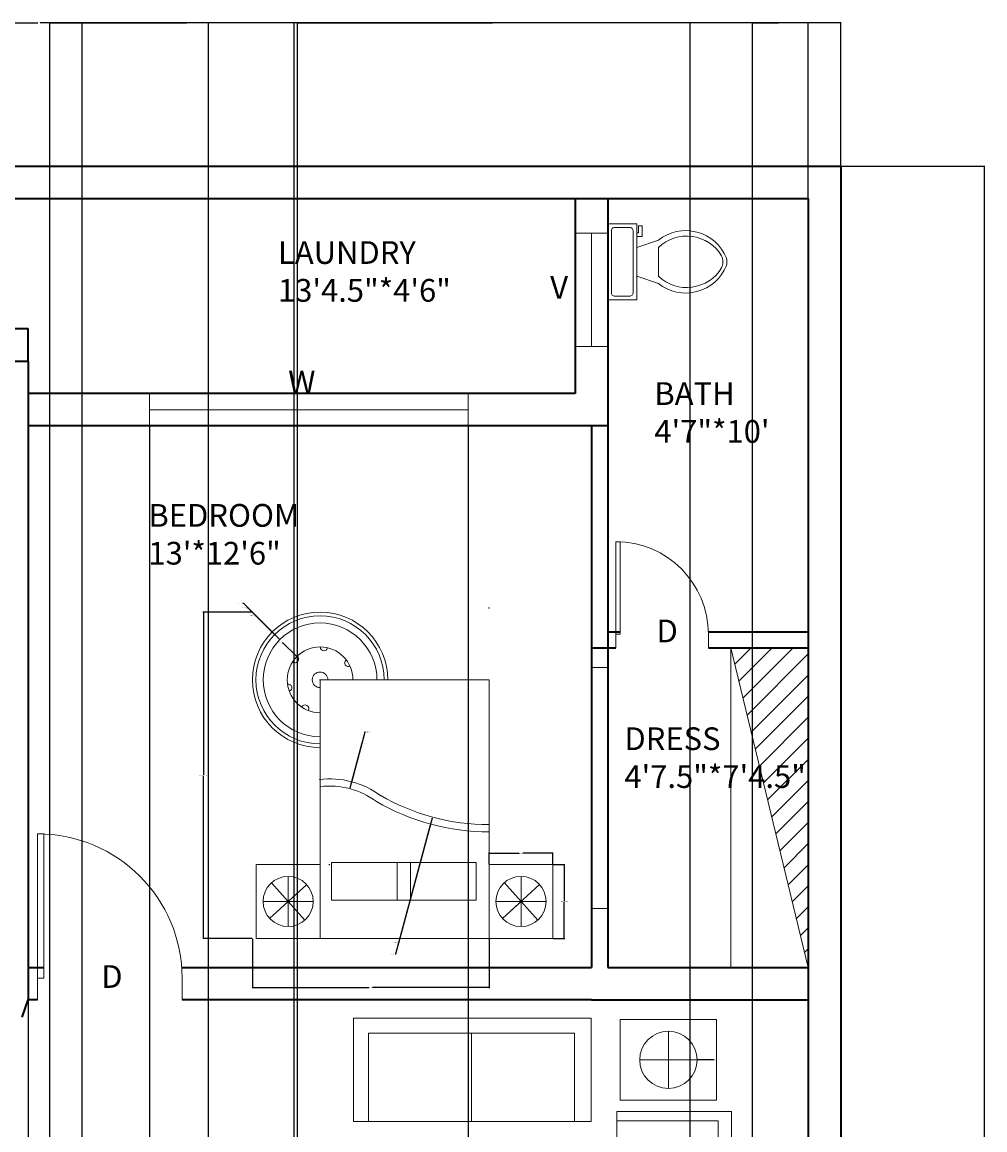
# Model space of a CAD drawing. Units: inches. Extents: x 2284 to 2815, y 1123 to 1948.
# Tile 6 of 6: x 2548 to 2814, y 1641 to 1948. Entities that reach past the tile are written whole.
import ezdxf

# ---------------------------------------------------------------- set-up
doc = ezdxf.new("R2010")
doc.units = ezdxf.units.IN
for name, color, linetype, lineweight in [('A-ANNO-DIMS', 2, 'Continuous', 18), ('A-AREA-IDEN', 30, 'Continuous', 18), ('A-CASE-PATT', 217, 'Continuous', 13), ('A-FLOR-CASE', 8, 'Continuous', 18), ('A-FLOR-FIXT', 9, 'Continuous', 18), ('A-WALL-PATT', 140, 'Continuous', 13), ('C-SITE-WALL', 7, 'Continuous', 35), ('DOOR', 190, 'Continuous', 18), ('FUR', 10, 'Continuous', 18), ('TEXT', 30, 'Continuous', 18), ('WALL', 7, 'Continuous', 35), ('WIND', 210, 'Continuous', 18)]:
    doc.layers.add(name, color=color, linetype=linetype, lineweight=lineweight)
doc.styles.get("Standard").update_dxf_attribs({"font": 'arial.ttf'})
doc.dimstyles.get("Standard").update_dxf_attribs({"dimtxt": 0.18, "dimasz": 0.18, "dimexe": 0.18, "dimexo": 0.0625, "dimgap": 0.09, "dimtad": 0, "dimtih": 1, "dimtoh": 1, "dimdec": 4, "dimzin": 0, "dimdsep": 46, "dimtxsty": 'Standard', "dimcen": 0.09, "dimadec": 0, "dimazin": 0, "dimtfac": 1, "dimtdec": 4, "dimtofl": 0, "dimtmove": 0, "dimatfit": 3, "dimfxl": 1, "dimtolj": 1, "dimtzin": 0, "dimarcsym": 0})

# ---------------------------------------------------------------- blocks, each defined once
blk = doc.blocks.new('*U2')
for p, q in [((0, 0), (0, -6)), ((40, 0), (40, -6))]:
    blk.add_line(p, q)
blk.add_lwpolyline([(0, 0), (0, 40), (1.75, 40), (1.75, 0)], close=True)
blk.add_arc((0, 0), 40, 0, 90)
blk = doc.blocks.new('*U4')
for p, q in [((9.5, -6), (9.5, -2)), ((-10, -8.5), (-8, -8.5)), ((-10, -9.5), (-10, -8.5)), ((-8, -8.5), (-8, -8)), ((-7, -8), (-7, -9.5)), ((-4, -8), (-6, -14)), ((4, -8), (6, -14)), ((-7, -9.5), (-10, -9.5)), ((4, -14), (-4, -14))]:
    blk.add_line(p, q)
blk.add_lwpolyline([(10.5, -8), (10.5, 0), (-10.5, 0), (-10.5, -8)], close=True)
for points in [[(-9.5, -2), (-9.5, -6)], [(8.5, -1), (-8.5, -1)], [(-8.5, -7), (8.5, -7)]]:
    blk.add_lwpolyline(points)
for centre, radius, start, end in [((-8.62, -1.88), 0.884, 81.8699, 188.1301), ((8.62, -1.88), 0.884, 351.8699, 98.1301), ((-8.62, -6.12), 0.884, 171.8699, 278.1301), ((8.62, -6.12), 0.884, 261.8699, 8.1301), ((3.52, -21.58), 12.17, 141.4691, 247.9714), ((4.2, -21.82), 11.33, 136.3677, 238.9468), ((-3.52, -21.58), 12.17, 292.0284, 38.5307), ((-4.2, -21.82), 11.33, 301.053, 43.6321), ((0, -27.88), 4, 245.7318, 294.2682), ((0, -29), 4, 254.8605, 285.1395)]:
    blk.add_arc(centre, radius, start, end)
blk = doc.blocks.new('BED-DOUBLE-WITH-RUG')
for points in [[(0, 0), (71.68, 0), (71.68, 46.8), (0, 46.8)], [(10.67, 21.75), (21.03, 21.75), (21.03, 43.61), (10.67, 43.61)], [(10.67, 3.58), (21.03, 3.58), (21.03, 25.43), (10.67, 25.43)]]:
    blk.add_lwpolyline(points, close=True)
for centre, radius, start, end in [((71.68, 46.8), 18.75, 270, 180), ((71.68, 46.8), 17.75, 270, 180), ((71.68, 46.8), 15.75, 270, 180), ((71.68, 46.8), 9.1, 270, 180), ((69.48, 55.63), 1, 197.1257, 10.8048), ((77.45, 53.83), 1.1, 144.137, 317.2027), ((63.62, 51.01), 1.12, 245.9164, 58.891), ((20.54, 44.16), 21.72, 323.3068, 6.9612), ((20.54, 44.16), 23.72, 323.3068, 6.9612), ((71.68, 46.8), 2.16, 270, 180), ((80.72, 45.75), 0.986, 86.4879, 260.2794), ((76.34, 38.98), 1, 33.9622, 207.6652), ((91.6, 0), 62.04, 149.8305, 180), ((91.6, 0), 60.04, 149.8305, 180)]:
    blk.add_arc(centre, radius, start, end)
blk = doc.blocks.new('NIGHTSTAND-LAMP')
for p, q in [((10.28, 1.89), (10.28, 15.8)), ((15.48, 13.46), (5.08, 4.23)), ((10.28, 8.85), (5.59, 13.98)), ((5.59, 13.98), (14.97, 3.71)), ((10.28, 8.85), (15.48, 13.46)), ((3.33, 8.85), (17.23, 8.85))]:
    blk.add_line(p, q)
blk.add_lwpolyline([(0, 0), (20.56, 0), (20.56, 17.69), (0, 17.69)], close=True)
blk.add_circle((10.28, 8.85), 6.95)
blk = doc.blocks.new('*D14')
at = {"layer": 'A-ANNO-DIMS', "color": 0, "lineweight": -2, "transparency": 16777216}
for p, q in [((2611.59, 1784.82), (2597.91, 1784.82)), ((2598.09, 1784.64), (2598.09, 1739.79)), ((2598.09, 1694.58), (2598.09, 1739.43)), ((2611.59, 1694.4), (2597.91, 1694.4))]:
    blk.add_line(p, q, dxfattribs=at)
at = {"layer": 'A-ANNO-DIMS', "color": 0, "transparency": 16777216}
for points in [[(2598.06, 1784.64), (2598.12, 1784.64), (2598.09, 1784.82)], [(2598.06, 1694.58), (2598.12, 1694.58), (2598.09, 1694.4)]]:
    blk.add_solid(points, dxfattribs=at)
at = {"layer": 'Defpoints', "color": 0, "transparency": 16777216}
for p in [(2598.09, 1784.82), (2611.65, 1784.82), (2611.65, 1694.4)]:
    blk.add_point(p, dxfattribs=at)
at = {"layer": 'A-ANNO-DIMS', "color": 0, "transparency": 16777216, "insert": (2598.09, 1739.61), "char_height": 0.18, "attachment_point": 5}
blk.add_mtext('\\A1;BED / RUG 90 TYP.', dxfattribs=at)
blk = doc.blocks.new('*D15')
at = {"layer": 'A-ANNO-DIMS', "color": 0, "lineweight": -2, "transparency": 16777216}
for p, q in [((2611.65, 1694.33), (2611.65, 1680.65)), ((2677.19, 1694.33), (2677.19, 1680.65)), ((2611.83, 1680.83), (2643.89, 1680.83)), ((2677.01, 1680.83), (2644.95, 1680.83))]:
    blk.add_line(p, q, dxfattribs=at)
at = {"layer": 'A-ANNO-DIMS', "color": 0, "transparency": 16777216}
for points in [[(2611.83, 1680.86), (2611.83, 1680.8), (2611.65, 1680.83)], [(2677.01, 1680.86), (2677.01, 1680.8), (2677.19, 1680.83)]]:
    blk.add_solid(points, dxfattribs=at)
at = {"layer": 'Defpoints', "color": 0, "transparency": 16777216}
for p in [(2611.65, 1694.4), (2677.19, 1694.4), (2611.65, 1680.83)]:
    blk.add_point(p, dxfattribs=at)
at = {"layer": 'A-ANNO-DIMS', "color": 0, "transparency": 16777216, "insert": (2644.42, 1680.83), "char_height": 0.18, "attachment_point": 5}
blk.add_mtext('\\A1;66 TYP.', dxfattribs=at)
blk = doc.blocks.new('*D16')
at = {"layer": 'A-ANNO-DIMS', "color": 0, "lineweight": -2, "transparency": 16777216}
for p, q in [((2694.94, 1714.96), (2698.15, 1714.96)), ((2697.97, 1714.78), (2697.97, 1704.86)), ((2697.97, 1694.58), (2697.97, 1704.49)), ((2694.94, 1694.4), (2698.15, 1694.4))]:
    blk.add_line(p, q, dxfattribs=at)
at = {"layer": 'A-ANNO-DIMS', "color": 0, "transparency": 16777216}
for points in [[(2697.94, 1714.78), (2698, 1714.78), (2697.97, 1714.96)], [(2697.94, 1694.58), (2698, 1694.58), (2697.97, 1694.4)]]:
    blk.add_solid(points, dxfattribs=at)
at = {"layer": 'Defpoints', "color": 0, "transparency": 16777216}
for p in [(2694.88, 1714.96), (2697.97, 1714.96), (2694.88, 1694.4)]:
    blk.add_point(p, dxfattribs=at)
at = {"layer": 'A-ANNO-DIMS', "color": 0, "transparency": 16777216, "insert": (2697.97, 1704.68), "char_height": 0.18, "attachment_point": 5}
blk.add_mtext('\\A1;NIGHTSTAND 21 TYP.', dxfattribs=at)
blk = doc.blocks.new('*D17')
at = {"layer": 'A-ANNO-DIMS', "color": 0, "lineweight": -2, "transparency": 16777216}
for p, q in [((2677.19, 1715.02), (2677.19, 1718.22)), ((2677.37, 1718.04), (2685.52, 1718.04)), ((2694.7, 1718.04), (2686.56, 1718.04)), ((2694.88, 1715.02), (2694.88, 1718.22))]:
    blk.add_line(p, q, dxfattribs=at)
at = {"layer": 'A-ANNO-DIMS', "color": 0, "transparency": 16777216}
for points in [[(2677.37, 1718.07), (2677.37, 1718.01), (2677.19, 1718.04)], [(2694.7, 1718.07), (2694.7, 1718.01), (2694.88, 1718.04)]]:
    blk.add_solid(points, dxfattribs=at)
at = {"layer": 'Defpoints', "color": 0, "transparency": 16777216}
for p in [(2677.19, 1718.04), (2677.19, 1714.96), (2694.88, 1714.96)]:
    blk.add_point(p, dxfattribs=at)
at = {"layer": 'A-ANNO-DIMS', "color": 0, "transparency": 16777216, "insert": (2686.04, 1718.04), "char_height": 0.18, "attachment_point": 5}
blk.add_mtext('\\A1;18 TYP.', dxfattribs=at)
blk = doc.blocks.new('*D20')
at = {"layer": 'A-ANNO-DIMS', "color": 0, "lineweight": -2, "transparency": 16777216}
for p, q in [((2330.55, 1908.47), (2330.55, 1948.28)), ((2330.73, 1948.1), (2552.26, 1948.1)), ((2774.37, 1948.1), (2552.85, 1948.1)), ((2774.55, 1908.47), (2774.55, 1948.28))]:
    blk.add_line(p, q, dxfattribs=at)
at = {"layer": 'A-ANNO-DIMS', "color": 0, "transparency": 16777216}
for points in [[(2330.73, 1948.13), (2330.73, 1948.07), (2330.55, 1948.1)], [(2774.37, 1948.13), (2774.37, 1948.07), (2774.55, 1948.1)]]:
    blk.add_solid(points, dxfattribs=at)
at = {"layer": 'Defpoints', "color": 0, "transparency": 16777216}
for p in [(2774.55, 1948.1), (2330.55, 1908.4), (2774.55, 1908.4)]:
    blk.add_point(p, dxfattribs=at)
at = {"layer": 'A-ANNO-DIMS', "color": 0, "transparency": 16777216, "insert": (2552.55, 1948.1), "char_height": 0.18, "attachment_point": 5}
blk.add_mtext('\\A1;444', dxfattribs=at)
blk = doc.blocks.new('*D21')
at = {"layer": 'A-ANNO-DIMS', "color": 0, "lineweight": -2, "transparency": 16777216}
for p, q in [((2774.62, 1908.4), (2814.43, 1908.4)), ((2814.25, 1908.22), (2814.25, 1542.59)), ((2814.25, 1176.58), (2814.25, 1542.22)), ((2774.62, 1176.4), (2814.43, 1176.4))]:
    blk.add_line(p, q, dxfattribs=at)
at = {"layer": 'A-ANNO-DIMS', "color": 0, "transparency": 16777216}
for points in [[(2814.22, 1908.22), (2814.28, 1908.22), (2814.25, 1908.4)], [(2814.22, 1176.58), (2814.28, 1176.58), (2814.25, 1176.4)]]:
    blk.add_solid(points, dxfattribs=at)
at = {"layer": 'Defpoints', "color": 0, "transparency": 16777216}
for p in [(2774.55, 1908.4), (2814.25, 1908.4), (2774.55, 1176.4)]:
    blk.add_point(p, dxfattribs=at)
at = {"layer": 'A-ANNO-DIMS', "color": 0, "transparency": 16777216, "insert": (2814.25, 1542.4), "char_height": 0.18, "attachment_point": 5}
blk.add_mtext('\\A1;732', dxfattribs=at)
blk = doc.blocks.new('*D43')
at = {"layer": 'A-ANNO-DIMS', "color": 0, "lineweight": -2, "transparency": 16777216}
for p, q in [((2564.55, 1368.47), (2564.55, 1948.28)), ((2564.73, 1948.1), (2593.47, 1948.1)), ((2623, 1948.1), (2594.26, 1948.1)), ((2623.18, 1368.47), (2623.18, 1948.28))]:
    blk.add_line(p, q, dxfattribs=at)
at = {"layer": 'A-ANNO-DIMS', "color": 0, "transparency": 16777216}
for points in [[(2564.73, 1948.13), (2564.73, 1948.07), (2564.55, 1948.1)], [(2623, 1948.13), (2623, 1948.07), (2623.18, 1948.1)]]:
    blk.add_solid(points, dxfattribs=at)
at = {"layer": 'Defpoints', "color": 0, "transparency": 16777216}
for p in [(2623.18, 1948.1), (2564.55, 1368.4), (2623.18, 1368.4)]:
    blk.add_point(p, dxfattribs=at)
at = {"layer": 'A-ANNO-DIMS', "color": 0, "transparency": 16777216, "insert": (2593.87, 1948.1), "char_height": 0.18, "attachment_point": 5}
blk.add_mtext('\\A1;58.62', dxfattribs=at)
blk = doc.blocks.new('*D44')
at = {"layer": 'A-ANNO-DIMS', "color": 0, "lineweight": -2, "transparency": 16777216}
for p, q in [((2583.19, 1836.34), (2583.19, 1136.52)), ((2671.4, 1836.34), (2671.4, 1136.52)), ((2583.37, 1136.7), (2626.92, 1136.7)), ((2671.22, 1136.7), (2627.67, 1136.7))]:
    blk.add_line(p, q, dxfattribs=at)
at = {"layer": 'A-ANNO-DIMS', "color": 0, "transparency": 16777216}
for points in [[(2583.37, 1136.73), (2583.37, 1136.67), (2583.19, 1136.7)], [(2671.22, 1136.73), (2671.22, 1136.67), (2671.4, 1136.7)]]:
    blk.add_solid(points, dxfattribs=at)
at = {"layer": 'Defpoints', "color": 0, "transparency": 16777216}
for p in [(2583.19, 1836.4), (2671.4, 1836.4), (2671.4, 1136.7)]:
    blk.add_point(p, dxfattribs=at)
at = {"layer": 'A-ANNO-DIMS', "color": 0, "transparency": 16777216, "insert": (2627.29, 1136.7), "char_height": 0.18, "attachment_point": 5}
blk.add_mtext('\\A1;88.21', dxfattribs=at)
blk = doc.blocks.new('*D45')
at = {"layer": 'A-ANNO-DIMS', "color": 0, "lineweight": -2, "transparency": 16777216}
for p, q in [((2549.55, 1836.34), (2549.55, 1136.52)), ((2583.19, 1836.34), (2583.19, 1136.52)), ((2549.73, 1136.7), (2565.91, 1136.7)), ((2583.01, 1136.7), (2566.84, 1136.7))]:
    blk.add_line(p, q, dxfattribs=at)
at = {"layer": 'A-ANNO-DIMS', "color": 0, "transparency": 16777216}
for points in [[(2549.73, 1136.73), (2549.73, 1136.67), (2549.55, 1136.7)], [(2583.01, 1136.73), (2583.01, 1136.67), (2583.19, 1136.7)]]:
    blk.add_solid(points, dxfattribs=at)
at = {"layer": 'Defpoints', "color": 0, "transparency": 16777216}
for p in [(2549.55, 1836.4), (2583.19, 1836.4), (2583.19, 1136.7)]:
    blk.add_point(p, dxfattribs=at)
at = {"layer": 'A-ANNO-DIMS', "color": 0, "transparency": 16777216, "insert": (2566.37, 1136.7), "char_height": 0.18, "attachment_point": 5}
blk.add_mtext('\\A1;33.635', dxfattribs=at)
blk = doc.blocks.new('*D48')
at = {"layer": 'A-ANNO-DIMS', "color": 0, "lineweight": -2, "transparency": 16777216}
for p, q in [((2624.18, 1533.47), (2624.18, 1948.28)), ((2624.36, 1948.1), (2678.14, 1948.1)), ((2732.7, 1948.1), (2678.91, 1948.1)), ((2732.88, 1533.47), (2732.88, 1948.28))]:
    blk.add_line(p, q, dxfattribs=at)
at = {"layer": 'A-ANNO-DIMS', "color": 0, "transparency": 16777216}
for points in [[(2624.36, 1948.13), (2624.36, 1948.07), (2624.18, 1948.1)], [(2732.7, 1948.13), (2732.7, 1948.07), (2732.88, 1948.1)]]:
    blk.add_solid(points, dxfattribs=at)
at = {"layer": 'Defpoints', "color": 0, "transparency": 16777216}
for p in [(2732.88, 1948.1), (2624.18, 1533.4), (2732.88, 1533.4)]:
    blk.add_point(p, dxfattribs=at)
at = {"layer": 'A-ANNO-DIMS', "color": 0, "transparency": 16777216, "insert": (2678.53, 1948.1), "char_height": 0.18, "attachment_point": 5}
blk.add_mtext('\\A1;108.7', dxfattribs=at)
blk = doc.blocks.new('*D52')
at = {"layer": 'A-ANNO-DIMS', "color": 0, "lineweight": -2, "transparency": 16777216}
for p, q in [((2750.11, 1389.06), (2750.11, 1948.28)), ((2750.29, 1948.1), (2757.37, 1948.1)), ((2765.37, 1948.1), (2758.29, 1948.1)), ((2765.55, 1368.47), (2765.55, 1948.28))]:
    blk.add_line(p, q, dxfattribs=at)
at = {"layer": 'A-ANNO-DIMS', "color": 0, "transparency": 16777216}
for points in [[(2750.29, 1948.13), (2750.29, 1948.07), (2750.11, 1948.1)], [(2765.37, 1948.13), (2765.37, 1948.07), (2765.55, 1948.1)]]:
    blk.add_solid(points, dxfattribs=at)
at = {"layer": 'Defpoints', "color": 0, "transparency": 16777216}
for p in [(2765.55, 1948.1), (2750.11, 1389), (2765.55, 1368.4)]:
    blk.add_point(p, dxfattribs=at)
at = {"layer": 'A-ANNO-DIMS', "color": 0, "transparency": 16777216, "insert": (2757.83, 1948.1), "char_height": 0.18, "attachment_point": 5}
blk.add_mtext('\\A1;15.448', dxfattribs=at)
blk = doc.blocks.new('*D54')
at = {"layer": 'A-ANNO-DIMS', "color": 0, "lineweight": -2, "transparency": 16777216}
for p, q in [((2555.55, 1490.27), (2555.55, 1948.28)), ((2555.73, 1948.1), (2577.07, 1948.1)), ((2599.35, 1948.1), (2578.01, 1948.1)), ((2599.53, 1533.47), (2599.53, 1948.28))]:
    blk.add_line(p, q, dxfattribs=at)
at = {"layer": 'A-ANNO-DIMS', "color": 0, "transparency": 16777216}
for points in [[(2555.73, 1948.13), (2555.73, 1948.07), (2555.55, 1948.1)], [(2599.35, 1948.13), (2599.35, 1948.07), (2599.53, 1948.1)]]:
    blk.add_solid(points, dxfattribs=at)
at = {"layer": 'Defpoints', "color": 0, "transparency": 16777216}
for p in [(2599.53, 1948.1), (2599.53, 1533.4), (2555.55, 1490.2)]:
    blk.add_point(p, dxfattribs=at)
at = {"layer": 'A-ANNO-DIMS', "color": 0, "transparency": 16777216, "insert": (2577.54, 1948.1), "char_height": 0.18, "attachment_point": 5}
blk.add_mtext('\\A1;43.975', dxfattribs=at)
blk = doc.blocks.new('*D61')
at = {"layer": 'A-ANNO-DIMS', "color": 0, "lineweight": -2, "transparency": 16777216}
for p, q in [((2677.19, 1785.91), (2677.19, 1786.09)), ((2677.1, 1786), (2677.28, 1786)), ((2651.36, 1690.15), (2661, 1725.91)), ((2651.18, 1690.15), (2651.36, 1690.15))]:
    blk.add_line(p, q, dxfattribs=at)
at = {"layer": 'A-ANNO-DIMS', "color": 0, "transparency": 16777216}
blk.add_solid([(2660.97, 1725.92), (2661.03, 1725.91), (2661.04, 1726.09)], dxfattribs=at)
at = {"layer": 'Defpoints', "color": 0, "transparency": 16777216}
for p in [(2677.19, 1786), (2661.04, 1726.09)]:
    blk.add_point(p, dxfattribs=at)
at = {"layer": 'A-ANNO-DIMS', "color": 0, "transparency": 16777216, "insert": (2650.5, 1690.15), "char_height": 0.18, "attachment_point": 5}
blk.add_mtext('\\A1;2X R62.04', dxfattribs=at)
blk = doc.blocks.new('*D62')
at = {"layer": 'A-ANNO-DIMS', "color": 0, "lineweight": -2, "transparency": 16777216}
for p, q in [((2677.19, 1785.91), (2677.19, 1786.09)), ((2677.1, 1786), (2677.28, 1786)), ((2652.19, 1693.23), (2661.52, 1727.85)), ((2652.01, 1693.23), (2652.19, 1693.23))]:
    blk.add_line(p, q, dxfattribs=at)
at = {"layer": 'A-ANNO-DIMS', "color": 0, "transparency": 16777216}
blk.add_solid([(2661.49, 1727.85), (2661.55, 1727.84), (2661.56, 1728.02)], dxfattribs=at)
at = {"layer": 'Defpoints', "color": 0, "transparency": 16777216}
for p in [(2677.19, 1786), (2661.56, 1728.02)]:
    blk.add_point(p, dxfattribs=at)
at = {"layer": 'A-ANNO-DIMS', "color": 0, "transparency": 16777216, "insert": (2651.33, 1693.23), "char_height": 0.18, "attachment_point": 5}
blk.add_mtext('\\A1;2X R60.04', dxfattribs=at)
blk = doc.blocks.new('*D63')
at = {"layer": 'A-ANNO-DIMS', "color": 0, "lineweight": -2, "transparency": 16777216}
for p, q in [((2642.77, 1751.62), (2639.16, 1738.04)), ((2642.95, 1751.62), (2642.77, 1751.62)), ((2632.94, 1714.94), (2633.12, 1714.94)), ((2633.03, 1714.85), (2633.03, 1715.03))]:
    blk.add_line(p, q, dxfattribs=at)
at = {"layer": 'A-ANNO-DIMS', "color": 0, "transparency": 16777216}
blk.add_solid([(2639.13, 1738.05), (2639.19, 1738.03), (2639.12, 1737.87)], dxfattribs=at)
at = {"layer": 'Defpoints', "color": 0, "transparency": 16777216}
for p in [(2639.12, 1737.87), (2633.03, 1714.94)]:
    blk.add_point(p, dxfattribs=at)
at = {"layer": 'A-ANNO-DIMS', "color": 0, "transparency": 16777216, "insert": (2643.69, 1751.62), "char_height": 0.18, "attachment_point": 5}
blk.add_mtext('\\A1;2X R23.724', dxfattribs=at)
blk = doc.blocks.new('*D64')
at = {"layer": 'A-ANNO-DIMS', "color": 0, "lineweight": -2, "transparency": 16777216}
for p, q in [((2641.95, 1748.53), (2638.65, 1736.11)), ((2642.13, 1748.53), (2641.95, 1748.53)), ((2632.94, 1714.94), (2633.12, 1714.94)), ((2633.03, 1714.85), (2633.03, 1715.03))]:
    blk.add_line(p, q, dxfattribs=at)
at = {"layer": 'A-ANNO-DIMS', "color": 0, "transparency": 16777216}
blk.add_solid([(2638.62, 1736.11), (2638.68, 1736.1), (2638.6, 1735.93)], dxfattribs=at)
at = {"layer": 'Defpoints', "color": 0, "transparency": 16777216}
for p in [(2638.6, 1735.93), (2633.03, 1714.94)]:
    blk.add_point(p, dxfattribs=at)
at = {"layer": 'A-ANNO-DIMS', "color": 0, "transparency": 16777216, "insert": (2642.87, 1748.53), "char_height": 0.18, "attachment_point": 5}
blk.add_mtext('\\A1;2X R21.724', dxfattribs=at)
blk = doc.blocks.new('*D65')
at = {"layer": 'A-ANNO-DIMS', "color": 0, "lineweight": -2, "transparency": 16777216}
for p, q in [((2609.01, 1787.29), (2609.19, 1787.29)), ((2609.19, 1787.29), (2617.01, 1779.46)), ((2630.31, 1766.08), (2630.49, 1766.08)), ((2630.4, 1765.99), (2630.4, 1766.17))]:
    blk.add_line(p, q, dxfattribs=at)
at = {"layer": 'A-ANNO-DIMS', "color": 0, "transparency": 16777216}
blk.add_solid([(2617.04, 1779.48), (2616.99, 1779.44), (2617.14, 1779.33)], dxfattribs=at)
at = {"layer": 'Defpoints', "color": 0, "transparency": 16777216}
for p in [(2617.14, 1779.33), (2630.4, 1766.08)]:
    blk.add_point(p, dxfattribs=at)
at = {"layer": 'A-ANNO-DIMS', "color": 0, "transparency": 16777216, "insert": (2608.26, 1787.29), "char_height": 0.18, "attachment_point": 5}
blk.add_mtext('\\A1;2X R18.747', dxfattribs=at)
blk = doc.blocks.new('*D66')
at = {"layer": 'A-ANNO-DIMS', "color": 0, "lineweight": -2, "transparency": 16777216}
for p, q in [((2610.14, 1786.15), (2610.32, 1786.15)), ((2610.32, 1786.15), (2617.72, 1778.75)), ((2630.31, 1766.08), (2630.49, 1766.08)), ((2630.4, 1765.99), (2630.4, 1766.17))]:
    blk.add_line(p, q, dxfattribs=at)
at = {"layer": 'A-ANNO-DIMS', "color": 0, "transparency": 16777216}
blk.add_solid([(2617.74, 1778.77), (2617.7, 1778.73), (2617.85, 1778.62)], dxfattribs=at)
at = {"layer": 'Defpoints', "color": 0, "transparency": 16777216}
for p in [(2617.85, 1778.62), (2630.4, 1766.08)]:
    blk.add_point(p, dxfattribs=at)
at = {"layer": 'A-ANNO-DIMS', "color": 0, "transparency": 16777216, "insert": (2609.39, 1786.15), "char_height": 0.18, "attachment_point": 5}
blk.add_mtext('\\A1;2X R17.747', dxfattribs=at)
blk = doc.blocks.new('*D67')
at = {"layer": 'A-ANNO-DIMS', "color": 0, "lineweight": -2, "transparency": 16777216}
for p, q in [((2612.4, 1783.89), (2612.58, 1783.89)), ((2612.58, 1783.89), (2619.13, 1777.34)), ((2630.31, 1766.08), (2630.49, 1766.08)), ((2630.4, 1765.99), (2630.4, 1766.17))]:
    blk.add_line(p, q, dxfattribs=at)
at = {"layer": 'A-ANNO-DIMS', "color": 0, "transparency": 16777216}
blk.add_solid([(2619.16, 1777.36), (2619.11, 1777.32), (2619.26, 1777.21)], dxfattribs=at)
at = {"layer": 'Defpoints', "color": 0, "transparency": 16777216}
for p in [(2619.26, 1777.21), (2630.4, 1766.08)]:
    blk.add_point(p, dxfattribs=at)
at = {"layer": 'A-ANNO-DIMS', "color": 0, "transparency": 16777216, "insert": (2611.66, 1783.89), "char_height": 0.18, "attachment_point": 5}
blk.add_mtext('\\A1;2X R15.747', dxfattribs=at)
blk = doc.blocks.new('*D68')
at = {"layer": 'A-ANNO-DIMS', "color": 0, "lineweight": -2, "transparency": 16777216}
for p, q in [((2619.92, 1776.37), (2620.1, 1776.37)), ((2620.1, 1776.37), (2623.83, 1772.64)), ((2630.31, 1766.08), (2630.49, 1766.08)), ((2630.4, 1765.99), (2630.4, 1766.17))]:
    blk.add_line(p, q, dxfattribs=at)
at = {"layer": 'A-ANNO-DIMS', "color": 0, "transparency": 16777216}
blk.add_solid([(2623.86, 1772.66), (2623.81, 1772.62), (2623.96, 1772.51)], dxfattribs=at)
at = {"layer": 'Defpoints', "color": 0, "transparency": 16777216}
for p in [(2623.96, 1772.51), (2630.4, 1766.08)]:
    blk.add_point(p, dxfattribs=at)
at = {"layer": 'A-ANNO-DIMS', "color": 0, "transparency": 16777216, "insert": (2619.4, 1776.37), "char_height": 0.18, "attachment_point": 5}
blk.add_mtext('\\A1;2X R9.1', dxfattribs=at)
blk = doc.blocks.new('*D71')
at = {"layer": 'A-ANNO-DIMS', "color": 0, "lineweight": -2, "transparency": 16777216}
for p, q in [((2726.74, 1660.79), (2726.92, 1660.79)), ((2726.83, 1660.7), (2726.83, 1660.88)), ((2739.52, 1660.79), (2734.94, 1660.79))]:
    blk.add_line(p, q, dxfattribs=at)
at = {"layer": 'A-ANNO-DIMS', "color": 0, "transparency": 16777216}
blk.add_solid([(2734.94, 1660.82), (2734.94, 1660.76), (2734.76, 1660.79)], dxfattribs=at)
at = {"layer": 'Defpoints', "color": 0, "transparency": 16777216}
for p in [(2718.9, 1660.79), (2734.76, 1660.79)]:
    blk.add_point(p, dxfattribs=at)
at = {"layer": 'A-ANNO-DIMS', "color": 0, "transparency": 16777216, "insert": (2740.01, 1660.79), "char_height": 0.18, "attachment_point": 5}
blk.add_mtext('\\A1;∅15.86', dxfattribs=at)

msp = doc.modelspace()

# ---------------------------------------------------------------- hatches: boundary and pattern name
at = {"layer": 'A-CASE-PATT'}
h = msp.add_hatch(dxfattribs=at)
h.set_pattern_fill('ANSI31', color=256, scale=1.3)
h.paths.add_polyline_path([(2765.554, 1774.904), (2744.1119, 1774.904), (2765.554, 1686.404)])
h.paths.add_polyline_path([(2540.554, 1854.404), (2485.054, 1854.404), (2485.054, 1837.4988)])
at = {"layer": 'A-WALL-PATT'}
h = msp.add_hatch(dxfattribs=at)
h.set_pattern_fill('AR-SAND', color=256, scale=8.5)
h.paths.add_polyline_path([(2339.554, 1899.404), (2375.554, 1899.404), (2765.554, 1899.404), (2765.554, 1185.404), (2549.3222, 1185.404), (2549.3222, 1176.404), (2774.554, 1176.404), (2774.554, 1908.404), (2330.554, 1908.404), (2330.554, 1176.404), (2349.4276, 1176.404), (2349.4276, 1185.404), (2339.554, 1185.404)])
h.paths.add_polyline_path([(2710.054, 1899.404), (2701.054, 1899.404), (2701.054, 1889.8374), (2710.054, 1889.8374)], flags=17)
h = msp.add_hatch(dxfattribs=at)
h.set_pattern_fill('AR-SAND', color=256, scale=8.5)
h.paths.add_polyline_path([(2549.554, 1863.404), (2375.554, 1863.404), (2375.554, 1840.6021), (2384.554, 1840.6021), (2384.554, 1854.404), (2480.554, 1854.404), (2549.554, 1854.404)])
h.paths.add_polyline_path([(2384.554, 1795.904), (2384.554, 1809.1528), (2375.554, 1809.1528), (2375.554, 1758.7416), (2384.554, 1758.7416)])
h.paths.add_polyline_path([(2549.554, 1836.404), (2549.554, 1854.404), (2540.554, 1854.404), (2540.554, 1800.404), (2485.054, 1800.404), (2485.054, 1802.7347), (2480.554, 1802.7347), (2480.554, 1800.404), (2384.554, 1800.404), (2384.554, 1795.904), (2485.054, 1795.904), (2540.554, 1795.904), (2540.554, 1678.5102), (2543.2164, 1676.3784), (2547.9, 1672.6283), (2549.554, 1677.404), (2549.554, 1795.904)])
h.paths.add_polyline_path([(2452.31, 1803.9815), (2480.7795, 1803.9815), (2480.7795, 1802.7347), (2452.2828, 1802.7347), (2452.2828, 1803.9815), (2452.31, 1803.9815, -0.39915744), (2480.554, 1831.2306), (2480.554, 1854.404), (2540.554, 1854.404), (2485.054, 1837.4988), (2485.054, 1831.2315), (2480.7795, 1831.2315, 0.40145271)], flags=17)
h.paths.add_polyline_path([(2583.189, 1845.404), (2549.554, 1845.404), (2549.554, 1836.404), (2583.189, 1836.404)])
h.paths.add_polyline_path([(2710.054, 1858.3882), (2701.054, 1858.3882), (2701.054, 1845.404), (2671.4007, 1845.404), (2671.4007, 1836.404), (2710.054, 1836.404)])
h.paths.add_polyline_path([(2710.054, 1836.404), (2705.554, 1836.404), (2705.554, 1774.904), (2710.054, 1774.904), (2710.054, 1779.404)])
h.paths.add_polyline_path([(2765.554, 1779.404), (2737.9116, 1779.404, -0.00645116), (2737.9201, 1778.7436), (2737.9201, 1774.904), (2765.554, 1774.904)])
h.paths.add_polyline_path([(2712.3231, 1778.7436), (2712.3231, 1779.404), (2710.054, 1779.404), (2710.054, 1774.904), (2712.3231, 1774.904)])
h.paths.add_polyline_path([(2710.054, 1774.904), (2705.554, 1774.904), (2705.554, 1769.4647), (2710.054, 1769.4647)])
h.paths.add_polyline_path([(2710.054, 1702.7233), (2705.554, 1702.7233), (2705.554, 1686.404), (2592.0733, 1686.404, -0.01876983), (2592.186, 1683.404), (2592.186, 1677.404), (2705.554, 1677.404), (2765.554, 1677.404), (2765.554, 1686.404), (2710.054, 1686.404)])
h.paths.add_polyline_path([(2384.554, 1641.404), (2375.554, 1641.404), (2375.554, 1637.3708), (2381.554, 1637.3708), (2384.554, 1637.3708)])
h.paths.add_polyline_path([(2384.554, 1678.0573), (2375.554, 1678.0573), (2375.554, 1641.404), (2384.554, 1641.404), (2522.8991, 1641.404), (2518.2155, 1645.1541, -0.00736412), (2517.3067, 1645.904), (2384.554, 1645.904)])
h.paths.add_polyline_path([(2384.554, 1597.4834, -0.01876983), (2381.554, 1597.3708), (2375.554, 1597.3708), (2375.554, 1591.564), (2384.554, 1591.564)])
h.paths.add_polyline_path([(2384.554, 1533.404), (2384.554, 1538.4896), (2375.554, 1538.4896), (2375.554, 1524.404), (2384.554, 1524.404)])
h.paths.add_polyline_path([(2506.054, 1533.404), (2506.054, 1598.7748), (2500.054, 1598.7748, -0.01876983), (2497.054, 1598.8874), (2497.054, 1533.404), (2384.554, 1533.404), (2384.554, 1524.404), (2497.054, 1524.404), (2506.054, 1524.404)])
h.paths.add_polyline_path([(2473.054, 1446.985), (2468.9674, 1446.985, -0.00379375), (2468.554, 1446.9881), (2468.554, 1428.404), (2473.054, 1428.404)])
h.paths.add_polyline_path([(2384.554, 1524.404), (2375.554, 1524.404), (2375.554, 1468.4232), (2384.554, 1468.4232)])
h.paths.add_polyline_path([(2473.054, 1480.904), (2384.554, 1480.904), (2384.554, 1476.404), (2468.554, 1476.404), (2468.554, 1474.2289), (2468.9674, 1474.2289), (2473.054, 1474.2289)])
h.paths.add_polyline_path([(2555.554, 1428.404), (2546.554, 1428.404), (2539.1317, 1428.404), (2539.1317, 1422.885), (2539.1317, 1419.404), (2546.554, 1419.404), (2555.554, 1419.404)])
h.paths.add_polyline_path([(2564.554, 1368.404), (2564.554, 1370.9838), (2561.554, 1370.9838), (2555.554, 1370.9838), (2555.554, 1359.404), (2564.554, 1359.404)])
h.paths.add_polyline_path([(2623.1768, 1368.404), (2564.554, 1368.404), (2564.554, 1359.404), (2623.1768, 1359.404)])
h.paths.add_polyline_path([(2492.7181, 1422.885), (2492.7181, 1428.404), (2384.554, 1428.404), (2384.554, 1440.6426), (2375.554, 1440.6426), (2375.554, 1419.404), (2492.7181, 1419.404)])
h.paths.add_polyline_path([(2765.554, 1368.404), (2710.406, 1368.404), (2710.406, 1359.404), (2765.554, 1359.404)])
h.paths.add_polyline_path([(2765.554, 1533.404), (2732.876, 1533.404), (2732.876, 1524.404), (2765.554, 1524.404)])
h.paths.add_polyline_path([(2624.1792, 1533.404), (2599.5288, 1533.404), (2590.3672, 1524.404), (2564.554, 1499.046), (2555.554, 1490.2048), (2555.554, 1410.9838), (2561.554, 1410.9838, -0.01876983), (2564.554, 1410.8712), (2564.554, 1486.4298), (2603.2099, 1524.404), (2624.1792, 1524.404)])
h.paths.add_polyline_path([(2555.554, 1490.2048), (2556.4043, 1491.0401), (2549.047, 1496.8538), (2545.7227, 1492.1958), (2543.8126, 1489.5193), (2555.554, 1480.2413)])
h.paths.add_polyline_path([(2514.6892, 1524.0031), (2506.054, 1530.8266), (2506.054, 1524.404), (2499.6656, 1524.404), (2500.474, 1523.7652), (2509.4548, 1516.6686), (2511.3649, 1519.3451)])
h.paths.add_polyline_path([(2365.9834, 1447.3726), (2374.9891, 1447.3726), (2374.9891, 1460.3342), (2365.9834, 1460.3342)], flags=9)
h.paths.add_polyline_path([(2366.9945, 1818.7713), (2376.0002, 1818.7713), (2376.0002, 1831.7328), (2366.9945, 1831.7328)], flags=9)
h.paths.add_polyline_path([(2363.2989, 1558.2059), (2374.7373, 1558.2059), (2374.7373, 1571.1674), (2363.2989, 1571.1674)], flags=9)
h.paths.add_polyline_path([(2364.8137, 1707.1012), (2376.2521, 1707.1012), (2376.2521, 1720.0627), (2364.8137, 1720.0627)], flags=9)
h.paths.add_polyline_path([(2460.3189, 1455.9932), (2469.8094, 1455.9932), (2469.8094, 1468.9547), (2460.3189, 1468.9547)], flags=9)
h.paths.add_polyline_path([(2558.6325, 1386.2225), (2568.1231, 1386.2225), (2568.1231, 1399.184), (2558.6325, 1399.184)], flags=9)
h.paths.add_polyline_path([(2378.5629, 1611.6816), (2388.0534, 1611.6816), (2388.0534, 1624.6431), (2378.5629, 1624.6431)], flags=9)
h.paths.add_polyline_path([(2490.2277, 1613.2326), (2499.7182, 1613.2326), (2499.7182, 1626.1941), (2490.2277, 1626.1941)], flags=9)
h.paths.add_polyline_path([(2522.9652, 1656.7942), (2532.4557, 1656.7942), (2532.4557, 1669.7557), (2522.9652, 1669.7557)], flags=9)
h.paths.add_polyline_path([(2567.5462, 1677.3031), (2577.0367, 1677.3031), (2577.0367, 1690.2646), (2567.5462, 1690.2646)], flags=9)
h.paths.add_polyline_path([(2363.196, 1676.9136), (2363.196, 1756.4461), (2350.2345, 1756.4461), (2350.2345, 1676.9136)], flags=9)
h.paths.add_polyline_path([(2515.5569, 1505.5998), (2535.7182, 1488.4964), (2539.8301, 1493.3434), (2519.6687, 1510.4468)], flags=9)
h.paths.add_polyline_path([(2503.6006, 1414.6146), (2530.0393, 1414.6146), (2530.0393, 1420.9707), (2503.6006, 1420.9707)], flags=9)
h.paths.add_polyline_path([(2391.2946, 1877.326), (2470.827, 1877.326), (2470.827, 1890.2876), (2391.2946, 1890.2876)], flags=9)
h.paths.add_polyline_path([(2580.3233, 1794.4386), (2629.1831, 1794.4386), (2629.1831, 1817.9089), (2580.3233, 1817.9089)], flags=9)
h.paths.add_polyline_path([(2585.6043, 1595.2228), (2648.3653, 1595.2228), (2648.3653, 1618.6931), (2585.6043, 1618.6931)], flags=9)
h.paths.add_polyline_path([(2591.9981, 1445.0189), (2637.889, 1445.0189), (2637.889, 1468.4892), (2591.9981, 1468.4892)], flags=9)
h.paths.add_polyline_path([(2459.0727, 1376.5795), (2515.4624, 1376.5795), (2515.4624, 1400.0498), (2459.0727, 1400.0498)], flags=9)
h.paths.add_polyline_path([(2481.8769, 1451.6363), (2543.2049, 1451.6363), (2543.2049, 1475.1066), (2481.8769, 1475.1066)], flags=9)
h.paths.add_polyline_path([(2470.0329, 1495.943), (2485.3842, 1495.943), (2485.3842, 1508.9045), (2470.0329, 1508.9045)], flags=9)
h.paths.add_polyline_path([(2419.5143, 1438.0898), (2446.0938, 1438.0898), (2446.0938, 1461.5344), (2419.5143, 1461.5344)], flags=9)
h.paths.add_polyline_path([(2425.6893, 1570.7133), (2467.4012, 1570.7133), (2467.4012, 1594.1836), (2425.6893, 1594.1836)], flags=25)
h.paths.add_polyline_path([(2428.101, 1758.2973), (2476.9609, 1758.2973), (2476.9609, 1781.7676), (2428.101, 1781.7676)], flags=25)

# ---------------------------------------------------------------- linework, layer by layer
at = {"layer": 'A-FLOR-CASE'}
for q in [(2744.1119, 1686.404), (2765.554, 1686.404)]:
    msp.add_line((2744.1119, 1774.904), q, dxfattribs=at)
at = {"layer": 'C-SITE-WALL'}
for p, q in [((2330.554, 1908.404), (2774.554, 1908.404)), ((2774.554, 1908.404), (2774.554, 1176.404)), ((2339.554, 1899.404), (2765.554, 1899.404)), ((2540.554, 1899.404), (2701.054, 1899.404)), ((2765.554, 1899.404), (2765.554, 1185.404))]:
    msp.add_line(p, q, dxfattribs=at)
at = {"layer": 'FUR'}
for p, q in [((2643.7617, 1643.7007), (2643.7617, 1668.1845)), ((2643.7617, 1668.1845), (2700.8479, 1668.1845)), ((2672.3048, 1668.1845), (2672.3048, 1643.7007)), ((2700.8479, 1668.1845), (2700.8479, 1643.7007)), ((2726.834, 1652.863), (2726.834, 1668.7244)), ((2718.9033, 1660.7937), (2734.7648, 1660.7937)), ((2740.6212, 1643.8812), (2712.5251, 1643.8812)), ((2740.6212, 1563.5556), (2740.6212, 1643.8812))]:
    msp.add_line(p, q, dxfattribs=at)
for points in [[(2705.4863, 1643.7007), (2639.6005, 1643.7007), (2639.6005, 1672.3422), (2705.4863, 1672.3422)], [(2713.4769, 1649.6478), (2740.1912, 1649.6478), (2740.1912, 1671.9396), (2713.4769, 1671.9396)], [(2744.3301, 1646.5004), (2712.5251, 1646.5004), (2712.5251, 1560.4509), (2744.3301, 1560.4509)]]:
    msp.add_lwpolyline(points, close=True, dxfattribs=at)
msp.add_circle((2726.834, 1660.7937), 7.9307, dxfattribs=at)
at = {"layer": 'WALL'}
for p, q in [((2701.054, 1899.404), (2701.054, 1863.404)), ((2701.054, 1899.404), (2701.054, 1845.404)), ((2710.054, 1899.404), (2710.054, 1836.404)), ((2710.054, 1899.404), (2710.054, 1779.404)), ((2375.554, 1863.404), (2549.554, 1863.404)), ((2549.554, 1854.404), (2549.554, 1863.404)), ((2384.554, 1854.404), (2549.554, 1854.404)), ((2549.554, 1854.404), (2549.554, 1795.904)), ((2701.054, 1845.404), (2549.554, 1845.404)), ((2710.054, 1836.404), (2549.554, 1836.404)), ((2549.554, 1836.404), (2549.554, 1686.404)), ((2705.554, 1836.404), (2705.554, 1774.904)), ((2549.554, 1795.904), (2549.554, 1677.404)), ((2710.054, 1779.404), (2713.443, 1779.404)), ((2710.054, 1779.404), (2710.054, 1774.904)), ((2737.9116, 1779.404), (2765.554, 1779.404)), ((2705.554, 1774.904), (2712.3231, 1774.904)), ((2705.554, 1774.904), (2705.554, 1686.404)), ((2710.054, 1774.904), (2710.054, 1686.404)), ((2737.9201, 1774.904), (2765.554, 1774.904)), ((2549.554, 1686.404), (2553.936, 1686.404)), ((2592.0733, 1686.404), (2705.554, 1686.404)), ((2710.054, 1686.404), (2765.554, 1686.404)), ((2547.9, 1672.6283), (2549.554, 1677.404)), ((2552.186, 1677.404), (2549.554, 1677.404)), ((2705.554, 1677.404), (2592.186, 1677.404)), ((2705.554, 1677.404), (2765.554, 1677.404)), ((2765.554, 1677.404), (2765.554, 1533.404))]:
    msp.add_line(p, q, dxfattribs=at)
at = {"layer": 'WIND'}
for p, q in [((2705.554, 1858.3882), (2705.554, 1889.8374)), ((2583.189, 1840.904), (2671.4007, 1840.904))]:
    msp.add_line(p, q, dxfattribs=at)
for points in [[(2710.054, 1889.8374), (2701.054, 1889.8374), (2701.054, 1858.3882), (2710.054, 1858.3882)], [(2583.189, 1836.404), (2671.4007, 1836.404), (2671.4007, 1845.404), (2583.189, 1845.404)], [(2705.554, 1769.4647), (2710.054, 1769.4647), (2710.054, 1702.7233), (2705.554, 1702.7233)]]:
    msp.add_lwpolyline(points, close=True, dxfattribs=at)

# ---------------------------------------------------------------- block references
at = {"layer": 'A-FLOR-FIXT', "xscale": -1, "rotation": 90}
msp.add_blockref('*U4', (2710.054, 1881.8863), dxfattribs=at)
at = {"layer": 'DOOR', "xscale": 0.639926597732846, "yscale": 0.639926597732846, "zscale": 0.639926597732846}
msp.add_blockref('*U2', (2712.3231, 1778.7436), dxfattribs=at)
at = {"layer": 'DOOR'}
msp.add_blockref('*U2', (2552.186, 1683.404), dxfattribs=at)
at = {"layer": 'FUR'}
for name, p, rotation in [('BED-DOUBLE-WITH-RUG', (2677.1919, 1694.3957), 90.00000000000122), ('NIGHTSTAND-LAMP', (2630.3969, 1694.3957), 89.99999999999834), ('NIGHTSTAND-LAMP', (2694.8823, 1694.3957), 89.99999999999547)]:
    msp.add_blockref(name, p, dxfattribs=dict(at, rotation=rotation))

# ---------------------------------------------------------------- texts
at = {"layer": 'A-AREA-IDEN', "attachment_point": 1}
for s, insert, char_height in [('LAUNDRY\\P13\'4.5"*4\'6"', (2618.7407, 1887.603), 6.289829), ('BATH\\P4\'7"*10\'', (2722.9472, 1848.5299), 6.28983), ('BEDROOM\\P13\'*12\'6"', (2582.8525, 1814.7833), 6.28983), ('DRESS\\P4\'7.5"*7\'4.5"', (2714.6536, 1752.9089), 6.289829)]:
    msp.add_mtext_dynamic_manual_height_columns(s, width=114.078767, gutter_width=31.4491, heights=[0], dxfattribs=dict(at, insert=insert, char_height=char_height))
at = {"layer": 'TEXT', "char_height": 6.2898, "attachment_point": 1}
for s, insert in [('V', (2694.1122, 1877.9275)), ('W', (2621.5584, 1851.6938)), ('D', (2723.5438, 1782.7602)), ('D', (2569.7966, 1687.0274))]:
    msp.add_mtext_dynamic_manual_height_columns(s, width=114.078767, gutter_width=31.4491, heights=[0], dxfattribs=dict(at, insert=insert))

# ---------------------------------------------------------------- dimensions: what is measured, and where the dimension line sits
at = {"layer": 'A-ANNO-DIMS'}
for base, p1, p2, override, picture, middle in [((2774.554, 1948.104), (2330.554, 1908.404), (2774.554, 1908.404), {"dimdec": 0, "dimlfac": 1, "dimrnd": 0, "dimzin": 0, "dimdsep": 46, "dimlunit": 2}, '*D20', (2552.554, 1948.104)), ((2599.5288, 1948.104), (2555.554, 1490.2048), (2599.5288, 1533.404), {"dimdec": 3, "dimlfac": 1, "dimrnd": 0, "dimzin": 0, "dimdsep": 46, "dimlunit": 2}, '*D54', (2577.5414, 1948.104)), ((2623.1768, 1948.104), (2564.554, 1368.404), (2623.1768, 1368.404), {"dimdec": 2, "dimlfac": 1, "dimrnd": 0, "dimzin": 0, "dimdsep": 46, "dimlunit": 2}, '*D43', (2593.8654, 1948.104)), ((2732.876, 1948.104), (2624.1792, 1533.404), (2732.876, 1533.404), {"dimdec": 1, "dimlfac": 1, "dimrnd": 0, "dimzin": 0, "dimdsep": 46, "dimlunit": 2}, '*D48', (2678.5276, 1948.104)), ((2765.554, 1948.104), (2750.1064, 1388.9955), (2765.554, 1368.404), {"dimdec": 3, "dimlfac": 1, "dimrnd": 0, "dimzin": 0, "dimdsep": 46, "dimlunit": 2}, '*D52', (2757.8302, 1948.104)), ((2583.189, 1136.704), (2549.554, 1836.404), (2583.189, 1836.404), {"dimdec": 3, "dimlfac": 1, "dimrnd": 0, "dimzin": 0, "dimdsep": 46, "dimlunit": 2}, '*D45', (2566.3715, 1136.704)), ((2671.4007, 1136.704), (2583.189, 1836.404), (2671.4007, 1836.404), {"dimdec": 2, "dimlfac": 1, "dimrnd": 0, "dimzin": 0, "dimdsep": 46, "dimlunit": 2}, '*D44', (2627.2949, 1136.704))]:
    dim = msp.add_linear_dim(base=base, p1=p1, p2=p2, dimstyle='Standard', override=override, dxfattribs=at)
    dim.commit()
    dim.dimension.update_dxf_attribs({"geometry": picture, "text_midpoint": middle})
dim = msp.add_linear_dim(base=(2814.254, 1908.404), p1=(2774.554, 1176.404), p2=(2774.554, 1908.404), angle=90, dimstyle='Standard', override={"dimdec": 0, "dimlfac": 1, "dimrnd": 0, "dimzin": 0, "dimdsep": 46, "dimlunit": 2}, dxfattribs=at)
dim.commit()
dim.dimension.update_dxf_attribs({"geometry": '*D21', "text_midpoint": (2814.254, 1542.404)})
for center, mpoint, override, picture, middle in [((2630.3969, 1766.07597), (2617.14115, 1779.33185), {"dimdec": 3, "dimlfac": 1, "dimrnd": 0, "dimzin": 0, "dimdsep": 46, "dimlunit": 2}, '*D65', (2608.26302, 1787.28537)), ((2630.3969, 1766.07597), (2617.84826, 1778.62474), {"dimdec": 3, "dimlfac": 1, "dimrnd": 0, "dimzin": 0, "dimdsep": 46, "dimlunit": 2}, '*D66', (2609.3944, 1786.154)), ((2677.1916, 1785.995), (2661.0449, 1726.0888), {"dimdec": 2, "dimlfac": 1, "dimrnd": 0, "dimzin": 0, "dimdsep": 46, "dimlunit": 2}, '*D61', (2650.5026, 1690.145)), ((2677.1916, 1785.995), (2661.565, 1728.02), {"dimdec": 2, "dimlfac": 1, "dimrnd": 0, "dimzin": 0, "dimdsep": 46, "dimlunit": 2}, '*D62', (2651.3346, 1693.2349)), ((2630.3969, 1766.07597), (2619.26197, 1777.21003), {"dimdec": 3, "dimlfac": 1, "dimrnd": 0, "dimzin": 0, "dimdsep": 46, "dimlunit": 2}, '*D67', (2611.65634, 1783.89046)), ((2630.3969, 1766.076), (2623.962, 1772.511), {"dimdec": 1, "dimlfac": 1, "dimrnd": 0, "dimzin": 0, "dimdsep": 46, "dimlunit": 2}, '*D68', (2619.4036, 1776.372)), ((2633.0298, 1714.9357), (2639.1169, 1737.8658), {"dimdec": 3, "dimlfac": 1, "dimrnd": 0, "dimzin": 0, "dimdsep": 46, "dimlunit": 2}, '*D63', (2643.6935, 1751.6238)), ((2633.0298, 1714.9357), (2638.603, 1735.9329), {"dimdec": 3, "dimlfac": 1, "dimrnd": 0, "dimzin": 0, "dimdsep": 46, "dimlunit": 2}, '*D64', (2642.8712, 1748.5313))]:
    dim = msp.add_radius_dim(center=center, mpoint=mpoint, text='2X <>', dimstyle='Standard', override=override, dxfattribs=at)
    dim.commit()
    dim.dimension.update_dxf_attribs({"geometry": picture, "text_midpoint": middle, "dimtype": 164})
for base, p1, p2, angle, text, picture, middle in [((2598.0863, 1784.8225), (2611.6504, 1694.3956), (2611.6504, 1784.8225), 90, 'BED / RUG <> TYP.', '*D14', (2598.0863, 1739.6091)), ((2677.1916, 1718.0416), (2694.8823, 1714.9573), (2677.1916, 1714.9573), 180, '<> TYP.', '*D17', (2686.0369, 1718.0416)), ((2697.9665, 1714.9573), (2694.8823, 1694.3956), (2694.8823, 1714.9573), 90, 'NIGHTSTAND <> TYP.', '*D16', (2697.9665, 1704.6765)), ((2611.6504, 1680.8316), (2677.1916, 1694.3956), (2611.6504, 1694.3956), 180, '<> TYP.', '*D15', (2644.421, 1680.8316))]:
    dim = msp.add_linear_dim(base=base, p1=p1, p2=p2, angle=angle, text=text, dimstyle='Standard', override={"dimdec": 0, "dimlfac": 1, "dimrnd": 0, "dimzin": 0, "dimdsep": 46, "dimlunit": 2}, dxfattribs=at)
    dim.commit()
    dim.dimension.update_dxf_attribs({"geometry": picture, "text_midpoint": middle})
dim = msp.add_diameter_dim_2p(p1=(2718.9033, 1660.7934), p2=(2734.7648, 1660.794), dimstyle='Standard', override={"dimdec": 2, "dimlfac": 1, "dimrnd": 0, "dimzin": 0, "dimdsep": 46, "dimlunit": 2}, dxfattribs=at)
dim.commit()
dim.dimension.update_dxf_attribs({"geometry": '*D71', "text_midpoint": (2739.5232, 1660.7942), "dimtype": 163})

doc.saveas('drawing.dxf')
